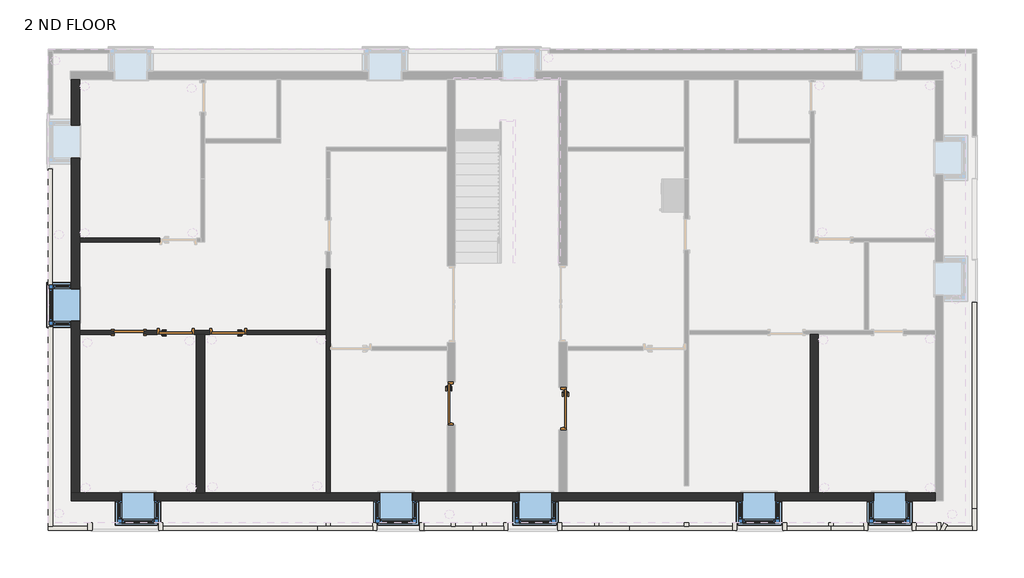
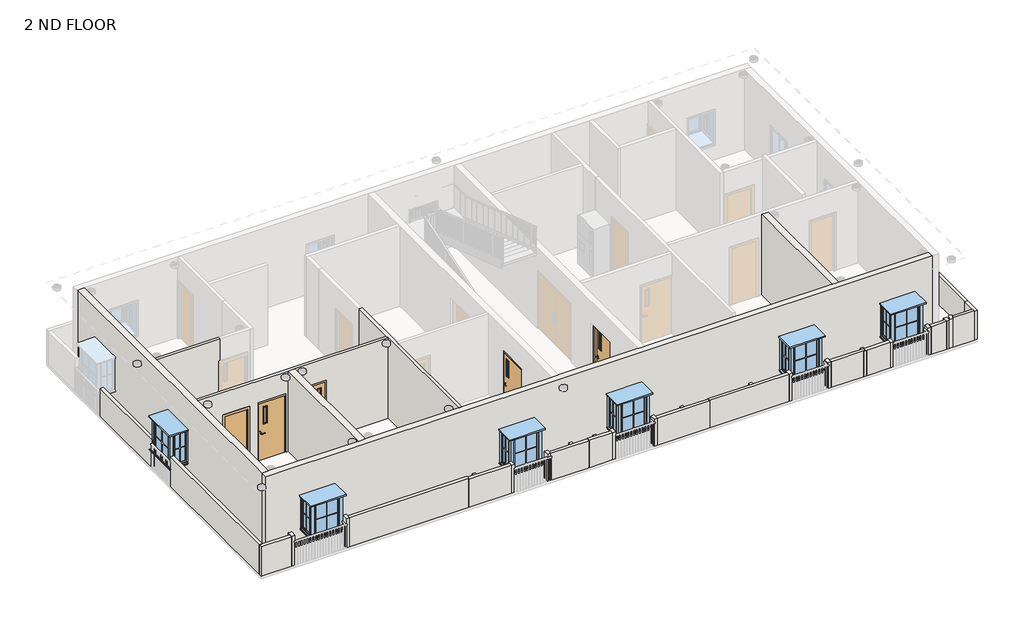
# One storey, part 1 of 7: 40 walls, 6 windows, 5 doors.
# Revit data of these elements (continued)
# Element 48 (IfcWindow, "Window-Bay-Casement-Box-90_Degree_Angle-Center_Fixed : 4'X3'")
#   Mark = "125"
#   Interior Trim Visibility = yes
#   Exterior Trim Visibility = yes
#   Phase Created = New Construction
#   Materials on its faces: "Clad - White", "Wood - Stained", "Glass"
# Element 49 (IfcWindow, "Window-Bay-Casement-Box-90_Degree_Angle-Center_Fixed : 4'X3'")
#   Mark = "126"
#   Interior Trim Visibility = yes
#   Exterior Trim Visibility = yes
#   Phase Created = New Construction
#   Materials on its faces: "Clad - White", "Wood - Stained", "Glass"
# Element 50 (IfcWindow, "Window-Bay-Casement-Box-90_Degree_Angle-Center_Fixed : 4'X3'")
#   Mark = "127"
#   Interior Trim Visibility = yes
#   Exterior Trim Visibility = yes
#   Phase Created = New Construction
#   Materials on its faces: "Clad - White", "Wood - Stained", "Glass"
# Element 51 (IfcWindow, "Window-Bay-Casement-Box-90_Degree_Angle-Center_Fixed : 4'X3'")
#   Mark = "130"
#   Interior Trim Visibility = yes
#   Exterior Trim Visibility = yes
#   Phase Created = New Construction
#   Materials on its faces: "Clad - White", "Wood - Stained", "Glass"
# Materials
#   "Wood - Birch": class "Wood", colour RGB 166 116 52, transparency 0, Cost = 0
#   "Glass": class "Glass", colour RGB 0 128 192, transparency 0.75, Description = "Soda Lime Glass", Cost = 0
#   "Metal - Paint Finish - Grey": class "Paint", colour RGB 104 104 104, transparency 0, Cost = 0
#   "Aluminum": class "Metal", colour RGB 247 247 247, transparency 0, Description = "Aluminum 6061", Cost = 0
#   "Door - Panel": class "Wood", colour RGB 210 159 95, transparency 0, Cost = 0
#   "Door - Frame": colour RGB 118 70 51, transparency 0, Cost = 0
#   "Concrete Masonry Units": class "Masonry", colour RGB 227 227 227, transparency 0, Description = "Concrete masonry units", Cost = 0
#   "Wood - Stained": class "Wood", colour RGB 224 178 126, transparency 0, Cost = 0
#   "Clad - White": class "Wood", colour RGB 242 242 238, transparency 0, Cost = 0
#   "Default Wall": colour RGB 128 128 128, transparency 0, Cost = 0
